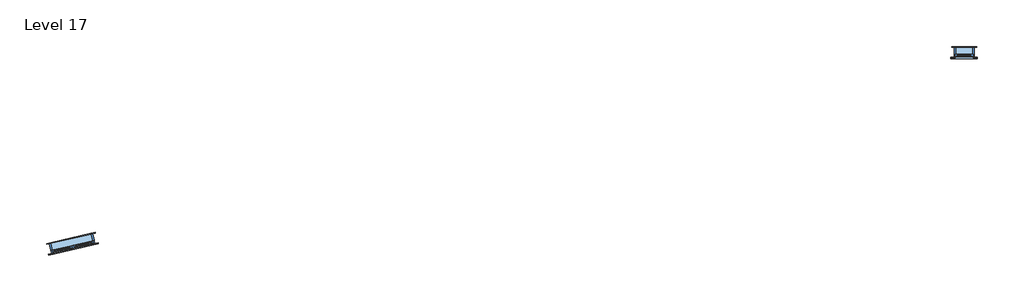
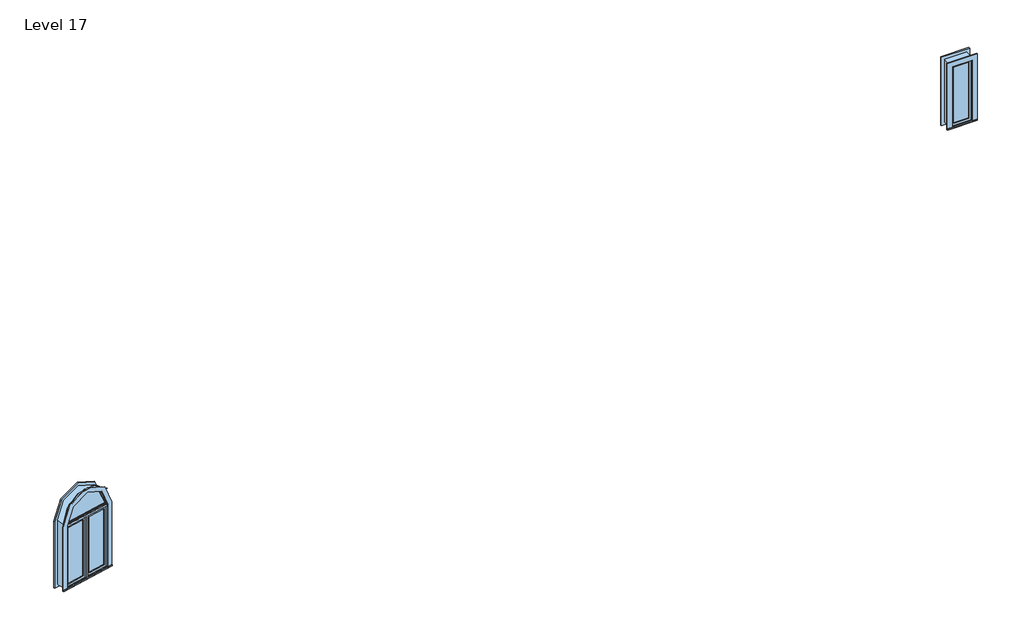
# One storey: 2 windows.
"""IFC4 building model written with IfcOpenShell, lengths in millimetres."""

from ifc_helpers import new_model, si_unit, origin, place, context, project, spatial, transform, mapped, element, save
from components import window_cf4adaea, window_a765b88f

model = new_model("IFC4")

# Units and contexts
model_context = context("Model", 3, world=origin())
ifc_project = project(units=[si_unit("LENGTHUNIT", "METRE", prefix="MILLI")], contexts=[model_context])

# Site, building, storey
site = spatial("IfcSite", under=ifc_project)
building = spatial("IfcBuilding", under=site)
storey = spatial("IfcBuildingStorey", under=building, Name="Level 17", Elevation=29565.6)

# Windows
placement = place(None, origin())
window_shape = window_cf4adaea(model_context)
element("IfcWindow", 1, ObjectType="36\" x 48\"", at=placement, inside=storey, context=model_context, shape_type="MappedRepresentation", body=[
    mapped(window_shape, transform((2569.5938084, -16298.3718892, 29565.6), x_axis=(-0.9741573207065573, -0.22587057026939494, 0.0), y_axis=(0.22587057026939494, -0.9741573207065573, 0.0), z_axis=(0.0, 0.0, 1.0))),
])
window_2_shape = window_a765b88f(model_context)
element("IfcWindow", 2, ObjectType="Awning with Trim : 16\" x 48\"", at=placement, inside=storey, context=model_context, shape_type="MappedRepresentation", body=[
    mapped(window_2_shape, transform((20968.614721, -12354.7237084, 29565.6), x_axis=(-1.0, 0.0, 0.0), y_axis=(0.0, -1.0, 0.0), z_axis=(0.0, 0.0, 1.0))),
])

save(model, "model.ifc")

# Revit data of these elements
# Type "36\" x 48\""
#   Type Mark = "38"
#   Construction Type Id = "SGL"
#   Assembly Code = "B2020100"
#   Analytic Construction = "Large single-glazed windows"
#   Visual Light Transmittance = 0.9
#   Solar Heat Gain Coefficient = 0.86
#   Heat Transfer Coefficient (U) = 0.979472 BTU/(h·ft²·°F)
#   Height = 4' - 0"
#   Default Sill Height = 3' - 0"
#   Trim Projection - Ext. = 0' - 0 1/2"
#   Trim Projection - Int. = 0' - 0 3/4"
#   Trim Width - Exterior = 0' - 3 1/2"
#   Trim Width - Interior = 0' - 3 1/2"
#   Width = 3' - 0"
#   Window Inset = 0' - 0 3/4"
#   Define Thermal Properties by = 1
#   Glass Pane Material = Glass
#   Sash Material = Sash
#   Trim Exterior Material = Trim
#   Trim Interior Material = Trim
#   Wall Closure = (empty or 0)
# Type "Awning with Trim : 16\" x 48\""
#   Type Mark = "14"
#   Construction Type Id = "GSP4R"
#   Assembly Code = "B2020100"
#   Analytic Construction = "1/8 in Pilkington single glazing"
#   Visual Light Transmittance = 0.9
#   Solar Heat Gain Coefficient = 0.78
#   Heat Transfer Coefficient (U) = 0.6496 BTU/(h·ft²·°F)
#   Height = 4' - 0"
#   Default Sill Height = 3' - 0"
#   Trim Projection - Ext. = 0' - 0 1/2"
#   Trim Projection - Int. = 0' - 0 3/4"
#   Trim Width - Exterior = 0' - 3 1/2"
#   Trim Width - Interior = 0' - 3 1/2"
#   Width = 1' - 4"
#   Window Inset = 0' - 0 3/4"
#   Define Thermal Properties by = 1
#   Glass Pane Material = Glass
#   Sash Material = Sash
#   Trim Exterior Material = Trim
#   Trim Interior Material = Trim
#   Wall Closure = (empty or 0)
# Element 1 (IfcWindow, "36\" x 48\"")
#   Mark = "25"
#   Phase Created = New Construction
#   Materials on its faces: "Sash", "Trim", "Glass"
# Element 2 (IfcWindow, "Awning with Trim : 16\" x 48\"")
#   Mark = "59"
#   Phase Created = New Construction
#   Materials on its faces: "Sash", "Trim", "Glass"
# Materials
#   "Glass": class "Glass", colour RGB 0 128 192, transparency 0.75, Description = "Soda Lime Glass", Cost = 0
#   "Sash": class "Wood", colour RGB 224 178 126, transparency 0
#   "Trim": class "Wood", colour RGB 224 178 126, transparency 0
